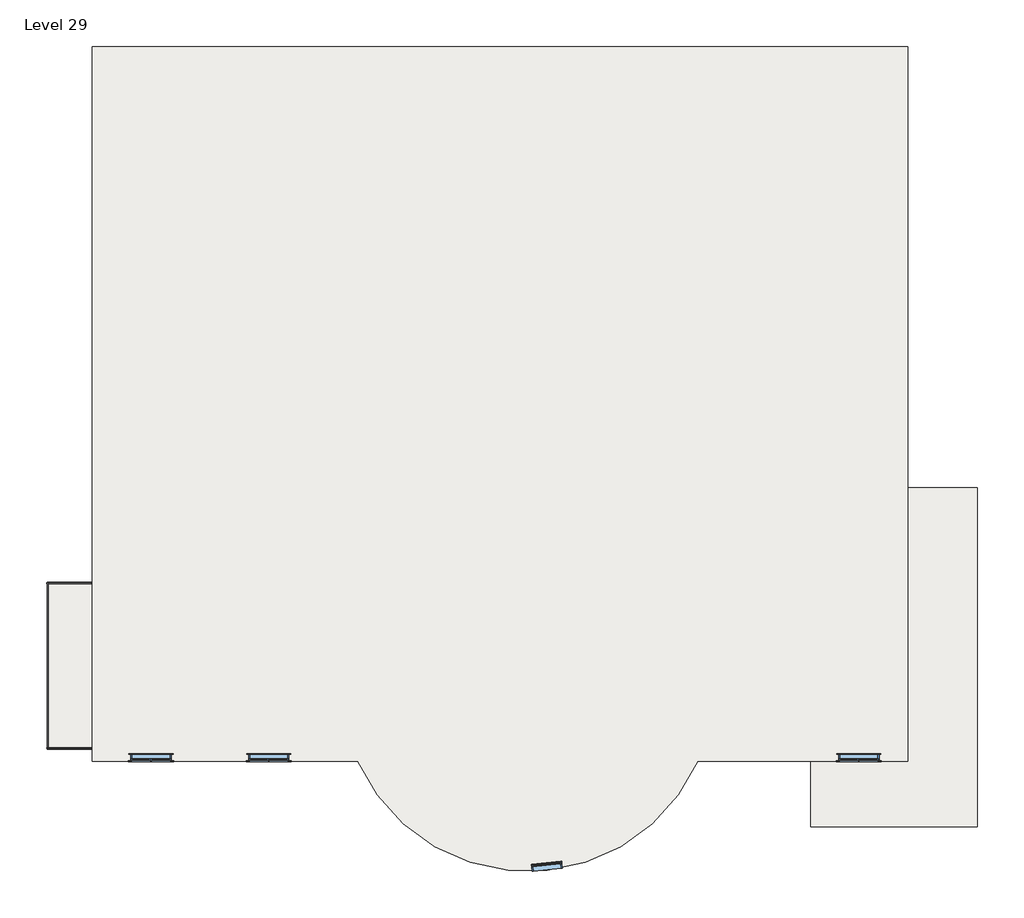
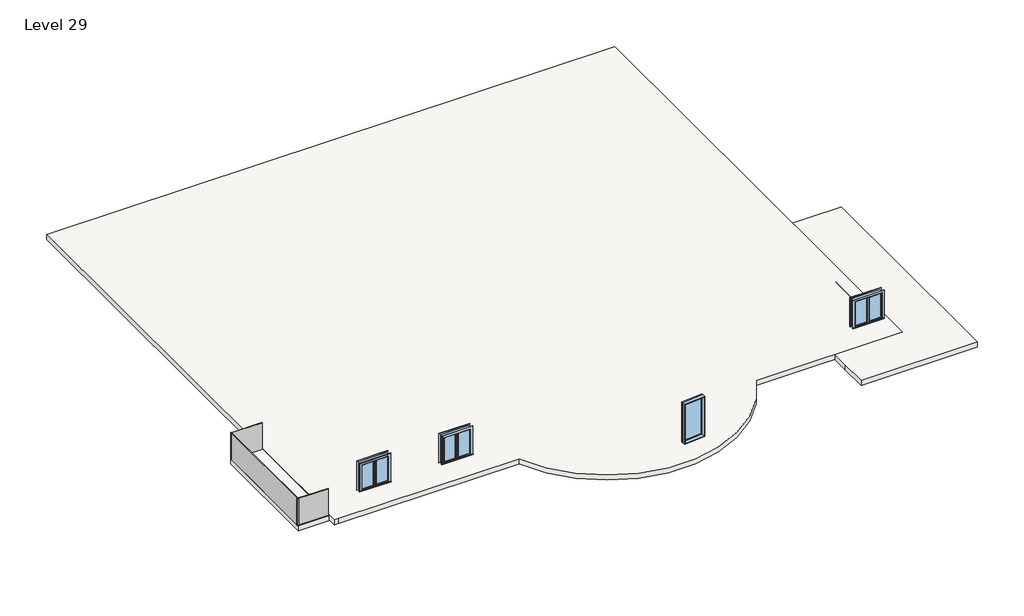
# One storey: 4 windows, 3 plates, 3 slabs.
"""IFC4 building model written with IfcOpenShell, lengths in millimetres."""

from ifc_helpers import new_model, si_unit, point, frame, frame_2d, origin, place, context, project, spatial, polyline, circle_curve, trimmed, segment, composite_curve, outline, extrude, transform, mapped, element, save
from components import system_panel_glazed_7d767388, system_panel_glazed_c55d8a5b, window_0862ab64, window_9a779fa2

model = new_model("IFC4")

# Units and contexts
model_context = context("Model", 3, world=origin())
ifc_project = project(units=[si_unit("LENGTHUNIT", "METRE", prefix="MILLI")], contexts=[model_context])

# Site, building, storey
site = spatial("IfcSite", under=ifc_project)
building = spatial("IfcBuilding", under=site)
storey = spatial("IfcBuildingStorey", under=building, Name="Level 29", Elevation=45872.4)

# Plates
placement = place(None, origin())
system_panel_glazed_shape = system_panel_glazed_7d767388(model_context)
element("IfcPlate", 1, ObjectType="System Panel : Glazed", at=placement, inside=storey, context=model_context, shape_type="MappedRepresentation", body=[
    mapped(system_panel_glazed_shape, transform((-17306.4505427, -8690.0239591, 45872.4), x_axis=(-1.0, 0.0, 0.0), y_axis=(0.0, -1.0, 0.0), z_axis=(0.0, 0.0, 1.0))),
])
element("IfcPlate", 2, ObjectType="System Panel : Glazed", at=placement, inside=storey, context=model_context, shape_type="MappedRepresentation", body=[
    mapped(system_panel_glazed_shape, transform((-17306.4505427, -13719.2239591, 45872.4), x_axis=(1.0, 0.0, 0.0), y_axis=(0.0, 1.0, 0.0), z_axis=(0.0, 0.0, 1.0))),
])
system_panel_glazed_2_shape = system_panel_glazed_c55d8a5b(model_context)
element("IfcPlate", 3, ObjectType="System Panel : Glazed", at=placement, inside=storey, context=model_context, shape_type="MappedRepresentation", body=[
    mapped(system_panel_glazed_2_shape, transform((-17979.5505427, -11204.6239591, 45872.4), x_axis=(0.0, -1.0, 0.0), y_axis=(1.0, 0.0, 0.0), z_axis=(0.0, 0.0, 1.0))),
])

# Slabs
element("IfcSlab", 4, ObjectType="9\"", at=placement, inside=storey, context=model_context, shape_type="SweptSolid", body=[
    extrude(outline(composite_curve([segment(polyline([(-16607.9505427, 7457.5128001), (7979.2494573, 7457.5128001), (7979.2494573, -14081.6871999), (1652.8739931, -14081.6871999)]), True, "CONTINUOUS"), segment(trimmed(circle_curve(frame_2d((-3476.1505427, -11791.9714001)), 5616.9111737), [point((1652.8739931, -14081.6871999))], [point((-8605.1750786, -14081.6871999))], False, "CARTESIAN"), True, "CONTINUOUS"), segment(polyline([(-8605.1750786, -14081.6871999), (-16404.7505427, -14081.6871999), (-16607.9505427, -14081.6871999), (-16607.9505427, 7457.5128001)]), True, "CONTINUOUS")], self_intersect=False)), frame((0.0, 0.0, 45650.3232641), z_axis=(0.0, 0.0, 1.0), x_axis=(1.0, 0.0, 0.0)), (0.0, 0.0, 1.0), 228.6),
])
element("IfcSlab", 5, ObjectType="9\"", at=placement, inside=storey, context=model_context, shape_type="SweptSolid", body=[
    extrude(outline(polyline([(-17953.126008, -8690.0239591), (-16581.526008, -8690.0239591), (-16581.526008, -13719.2239591), (-17953.126008, -13719.2239591), (-17953.126008, -8690.0239591)])), frame((0.0, 0.0, 45643.8), z_axis=(0.0, 0.0, 1.0), x_axis=(1.0, 0.0, 0.0)), (0.0, 0.0, 1.0), 228.6),
])
element("IfcSlab", 6, ObjectType="9\"", at=placement, inside=storey, context=model_context, shape_type="SweptSolid", body=[
    extrude(outline(polyline([(5053.3049901, -14840.0808221), (5053.3049901, -14078.0808221), (7237.7049901, -14078.0808221), (7440.9049901, -14078.0808221), (7440.9049901, -5848.4808221), (10082.5049901, -5848.4808221), (10082.5049901, -14840.0808221), (10082.5049901, -16059.2808221), (5053.3049901, -16059.2808221), (5053.3049901, -14840.0808221)])), frame((0.0, 0.0, 45643.8), z_axis=(0.0, 0.0, 1.0), x_axis=(1.0, 0.0, 0.0)), (0.0, 0.0, 1.0), 228.6),
])

# Windows
window_shape = window_0862ab64(model_context)
element("IfcWindow", 7, ObjectType="Casement Dbl with Trim : 48\" x 48\"", at=placement, inside=storey, context=model_context, shape_type="MappedRepresentation", body=[
    mapped(window_shape, transform((-14829.9505427, -13957.4308221, 45872.4), x_axis=(-1.0, 0.0, 0.0), y_axis=(0.0, -1.0, 0.0), z_axis=(0.0, 0.0, 1.0))),
])
element("IfcWindow", 8, ObjectType="Casement Dbl with Trim : 48\" x 48\"", at=placement, inside=storey, context=model_context, shape_type="MappedRepresentation", body=[
    mapped(window_shape, transform((-11282.0382271, -13957.4308221, 45872.4), x_axis=(-1.0, 0.0, 0.0), y_axis=(0.0, -1.0, 0.0), z_axis=(0.0, 0.0, 1.0))),
])
element("IfcWindow", 9, ObjectType="Casement Dbl with Trim : 48\" x 48\"", at=placement, inside=storey, context=model_context, shape_type="MappedRepresentation", body=[
    mapped(window_shape, transform((6506.0494573, -13957.4308221, 45872.4), x_axis=(-1.0, 0.0, 0.0), y_axis=(0.0, -1.0, 0.0), z_axis=(0.0, 0.0, 1.0))),
])
window_2_shape = window_9a779fa2(model_context)
element("IfcWindow", 10, ObjectType="Fixed : 36\" x 72\"", at=placement, inside=storey, context=model_context, shape_type="MappedRepresentation", body=[
    mapped(window_2_shape, transform((-2862.4706837, -17250.0995626, 46400.3772014), x_axis=(0.9944969265536162, 0.10476575335199584, 0.0), y_axis=(-0.10476575335199584, 0.9944969265536162, 0.0), z_axis=(0.0, 0.0, 1.0))),
])

save(model, "model.ifc")

# Revit data of these elements
# Type "System Panel : Glazed"
#   Construction Type Id = "GSP4R"
#   Analytic Construction = "1/8 in Pilkington single glazing"
#   Visual Light Transmittance = 0.9
#   Solar Heat Gain Coefficient = 0.86
#   Heat Transfer Coefficient (U) = 1.18115 BTU/(h·ft²·°F)
# Type "9\""
#   Assembly Code = "B1010"
#   Function = 0
#   Layers, outside or top first: 0' - 9" no material (function 1)
# Type "Casement Dbl with Trim : 48\" x 48\""
#   Type Mark = "10"
#   Construction Type Id = "GSP4R"
#   Assembly Code = "B2020100"
#   Analytic Construction = "1/8 in Pilkington single glazing"
#   Visual Light Transmittance = 0.9
#   Solar Heat Gain Coefficient = 0.78
#   Heat Transfer Coefficient (U) = 0.6496 BTU/(h·ft²·°F)
#   Height = 4' - 0"
#   Default Sill Height = 3' - 0"
#   Trim Projection - Ext. = 0' - 0 1/2"
#   Trim Projection - Int. = 0' - 0 3/4"
#   Trim Width - Exterior = 0' - 3 1/2"
#   Trim Width - Interior = 0' - 3 1/2"
#   Width = 4' - 0"
#   Window Inset = 0' - 0 3/4"
#   Define Thermal Properties by = 1
#   Glass Pane Material = Glass
#   Sash Material = Sash
#   Trim Exterior Material = Trim
#   Trim Interior Material = Trim
#   Wall Closure = (empty or 0)
# Type "Fixed : 36\" x 72\""
#   Type Mark = "9"
#   Construction Type Id = "GSP4R"
#   Assembly Code = "B2020100"
#   Analytic Construction = "1/8 in Pilkington single glazing"
#   Visual Light Transmittance = 0.9
#   Solar Heat Gain Coefficient = 0.78
#   Heat Transfer Coefficient (U) = 0.6496 BTU/(h·ft²·°F)
#   Height = 6' - 0"
#   Default Sill Height = 1' - 0"
#   Width = 3' - 0"
#   Window Inset = 0' - 0 3/4"
#   Define Thermal Properties by = 1
#   Glass Pane Material = Glass
#   Sash Material = Sash
#   Wall Closure = (empty or 0)
# Elements 1, 2, 3 (IfcPlate, "System Panel : Glazed")
#   Phase Created = New Construction
#   Materials on its faces: "Glass"
# Element 4 (IfcSlab, "9\"")
#   built-in parameter 1001955 = 1.5708 (stored number, unit not read)
#   Height Offset From Level = 0' - 0.25682"
#   Phase Created = New Construction
#   Materials on its faces: "Default Floor"
# Element 5 (IfcSlab, "9\"")
#   built-in parameter 1001955 = 3.14159 (stored number, unit not read)
#   Height Offset From Level = 0' - 0"
#   Phase Created = New Construction
#   Materials on its faces: "Default Floor"
# Element 6 (IfcSlab, "9\"")
#   built-in parameter 1001955 = -1.5708 (stored number, unit not read)
#   Height Offset From Level = 0' - 0"
#   Phase Created = New Construction
#   Materials on its faces: "Default Floor"
# Element 7 (IfcWindow, "Casement Dbl with Trim : 48\" x 48\"")
#   Mark = "19"
#   Phase Created = New Construction
#   Materials on its faces: "Sash", "Trim", "Glass"
# Element 8 (IfcWindow, "Casement Dbl with Trim : 48\" x 48\"")
#   Mark = "20"
#   Phase Created = New Construction
#   Materials on its faces: "Sash", "Trim", "Glass"
# Element 9 (IfcWindow, "Casement Dbl with Trim : 48\" x 48\"")
#   Mark = "47"
#   Phase Created = New Construction
#   Materials on its faces: "Sash", "Trim", "Glass"
# Element 10 (IfcWindow, "Fixed : 36\" x 72\"")
#   Mark = "2"
#   Phase Created = New Construction
#   Materials on its faces: "Sash", "Glass"
# Materials
#   "Glass": class "Glass", colour RGB 0 128 192, transparency 0.75, Description = "Soda Lime Glass", Cost = 0
#   "Sash": class "Wood", colour RGB 224 178 126, transparency 0
#   "Trim": class "Wood", colour RGB 224 178 126, transparency 0
#   "Default Floor": colour RGB 128 128 128, transparency 0
